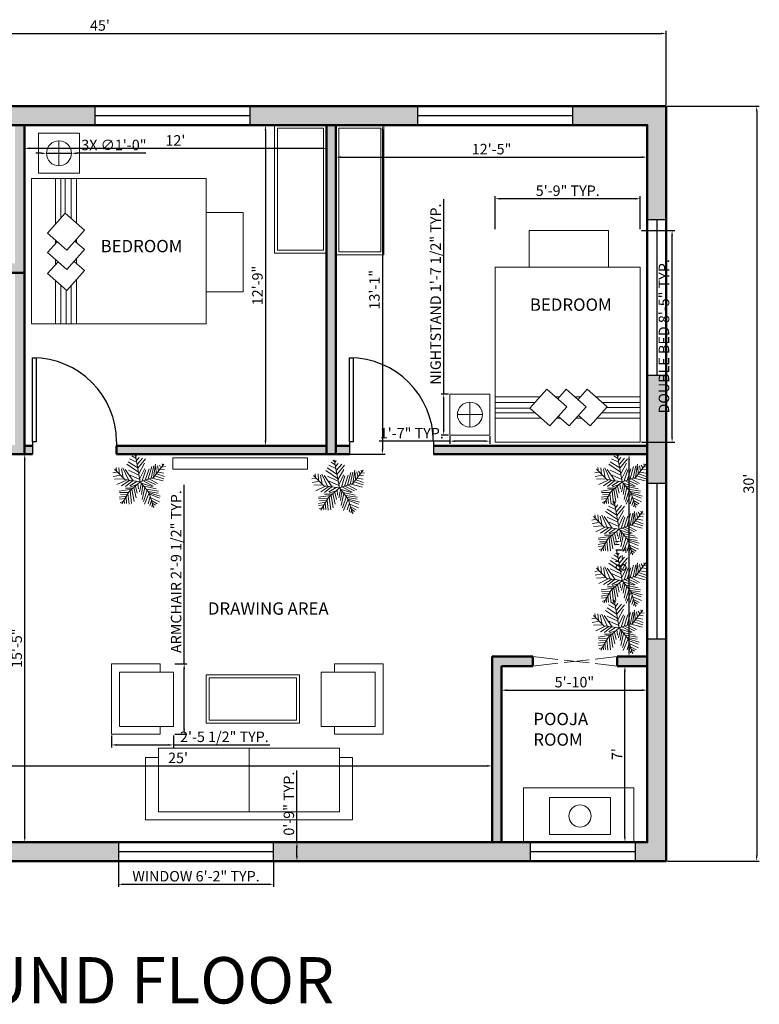
# Model space of a CAD drawing. Units: inches. Extents: x 1882 to 2467, y 1298 to 1767.
# Tile 2 of 2: x 2114 to 2467, y 1298 to 1767. Entities that reach past the tile are written whole.
import ezdxf

# ---------------------------------------------------------------- set-up
doc = ezdxf.new("R2010")
doc.units = ezdxf.units.IN
doc.linetypes.add('ACAD_ISO02W100', pattern=[15, 12, -3])
for name, color, linetype, lineweight in [('A-ANNO-DIMS', 2, 'Continuous', 18), ('A-ANNO-TEXT', 7, 'Continuous', 35), ('A-AREA-IDEN', 7, 'Continuous', 25), ('A-FURN', 8, 'Continuous', 18), ('A-WALL-OVHD', 160, 'ACAD_ISO02W100', 18), ('A-WALL-PATT', 160, 'Continuous', 13), ('DOOR', 140, 'Continuous', 25), ('TREE', 80, 'Continuous', 13), ('WALL', 160, 'Continuous', 50), ('WIND', 52, 'Continuous', 25)]:
    doc.layers.add(name, color=color, linetype=linetype, lineweight=lineweight)
doc.styles.get("Standard").update_dxf_attribs({"font": 'arial.ttf'})
doc.dimstyles.new('ISO-25', dxfattribs={"dimtxt": 5, "dimasz": 2.5, "dimexe": 1.25, "dimexo": 0.625, "dimtad": 1, "dimdec": 0, "dimlunit": 4, "dimtxsty": 'Standard', "dimcen": 2.5, "dimadec": 0, "dimazin": 0, "dimtfac": 1, "dimtdec": 0, "dimtmove": 0, "dimatfit": 3, "dimfxl": 1, "dimarcsym": 0})

# ---------------------------------------------------------------- blocks, each defined once
blk = doc.blocks.new('*U2')
for p, q in [((0, 0), (0, -6)), ((40, 0), (40, -6))]:
    blk.add_line(p, q)
blk.add_lwpolyline([(0, 0), (0, 40), (1.75, 40), (1.75, 0)], close=True)
blk.add_arc((0, 0), 40, 0, 90)
blk = doc.blocks.new('*D11')
at = {"layer": 'A-ANNO-DIMS', "color": 0, "lineweight": -2, "transparency": 16777216}
for p, q in [((2116.22, 1716.45), (2116.22, 1704.74)), ((2260.22, 1716.45), (2260.22, 1704.74)), ((2118.72, 1705.99), (2257.72, 1705.99))]:
    blk.add_line(p, q, dxfattribs=at)
at = {"layer": 'A-ANNO-DIMS', "color": 0, "lineweight": 100, "transparency": 16777216}
for points in [[(2118.72, 1706.41), (2118.72, 1705.57), (2116.22, 1705.99)], [(2257.72, 1706.41), (2257.72, 1705.57), (2260.22, 1705.99)]]:
    blk.add_solid(points, dxfattribs=at)
at = {"layer": 'Defpoints', "color": 0, "lineweight": 100, "transparency": 16777216}
for p in [(2116.22, 1717.07), (2260.22, 1717.07), (2260.22, 1705.99)]:
    blk.add_point(p, dxfattribs=at)
at = {"layer": 'A-ANNO-DIMS', "color": 0, "transparency": 16777216, "insert": (2188.22, 1709.12), "char_height": 5, "attachment_point": 5}
blk.add_mtext("12'", dxfattribs=at)
blk = doc.blocks.new('*D12')
at = {"layer": 'A-ANNO-DIMS', "color": 0, "lineweight": -2, "transparency": 16777216}
for p, q in [((2259.59, 1717.07), (2229.92, 1717.07)), ((2231.17, 1714.57), (2231.17, 1566.57)), ((2259.59, 1564.07), (2229.92, 1564.07))]:
    blk.add_line(p, q, dxfattribs=at)
at = {"layer": 'A-ANNO-DIMS', "color": 0, "lineweight": 100, "transparency": 16777216}
for points in [[(2230.75, 1714.57), (2231.58, 1714.57), (2231.17, 1717.07)], [(2230.75, 1566.57), (2231.58, 1566.57), (2231.17, 1564.07)]]:
    blk.add_solid(points, dxfattribs=at)
at = {"layer": 'Defpoints', "color": 0, "lineweight": 100, "transparency": 16777216}
for p in [(2260.22, 1717.07), (2231.17, 1564.07), (2260.22, 1564.07)]:
    blk.add_point(p, dxfattribs=at)
at = {"layer": 'A-ANNO-DIMS', "color": 0, "transparency": 16777216, "insert": (2227.99, 1640.57), "char_height": 5, "attachment_point": 5, "rotation": 90}
blk.add_mtext('12\'-9"', dxfattribs=at)
blk = doc.blocks.new('*D13')
at = {"layer": 'A-ANNO-DIMS', "color": 0, "lineweight": -2, "transparency": 16777216}
for p, q in [((2264.72, 1716.45), (2264.72, 1700.54)), ((2413.22, 1716.45), (2413.22, 1700.54)), ((2267.22, 1701.79), (2410.72, 1701.79))]:
    blk.add_line(p, q, dxfattribs=at)
at = {"layer": 'A-ANNO-DIMS', "color": 0, "lineweight": 100, "transparency": 16777216}
for points in [[(2267.22, 1702.21), (2267.22, 1701.38), (2264.72, 1701.79)], [(2410.72, 1702.21), (2410.72, 1701.38), (2413.22, 1701.79)]]:
    blk.add_solid(points, dxfattribs=at)
at = {"layer": 'Defpoints', "color": 0, "lineweight": 100, "transparency": 16777216}
for p in [(2264.72, 1717.07), (2413.22, 1717.07), (2413.22, 1701.79)]:
    blk.add_point(p, dxfattribs=at)
at = {"layer": 'A-ANNO-DIMS', "color": 0, "transparency": 16777216, "insert": (2338.97, 1704.97), "char_height": 5, "attachment_point": 5}
blk.add_mtext('12\'-5"', dxfattribs=at)
blk = doc.blocks.new('*D14')
at = {"layer": 'A-ANNO-DIMS', "color": 0, "lineweight": -2, "transparency": 16777216}
for p, q in [((2265.34, 1717.07), (2288.2, 1717.07)), ((2286.95, 1714.57), (2286.95, 1562.57)), ((2265.34, 1560.07), (2288.2, 1560.07))]:
    blk.add_line(p, q, dxfattribs=at)
at = {"layer": 'A-ANNO-DIMS', "color": 0, "lineweight": 100, "transparency": 16777216}
for points in [[(2286.53, 1714.57), (2287.36, 1714.57), (2286.95, 1717.07)], [(2286.53, 1562.57), (2287.36, 1562.57), (2286.95, 1560.07)]]:
    blk.add_solid(points, dxfattribs=at)
at = {"layer": 'Defpoints', "color": 0, "lineweight": 100, "transparency": 16777216}
for p in [(2264.72, 1717.07), (2264.72, 1560.07), (2286.95, 1560.07)]:
    blk.add_point(p, dxfattribs=at)
at = {"layer": 'A-ANNO-DIMS', "color": 0, "transparency": 16777216, "insert": (2283.77, 1638.57), "char_height": 5, "attachment_point": 5, "rotation": 90}
blk.add_mtext('13\'-1"', dxfattribs=at)
blk = doc.blocks.new('*D15')
at = {"layer": 'A-ANNO-DIMS', "color": 0, "lineweight": -2, "transparency": 16777216}
for p, q in [((2343.72, 1458.45), (2343.72, 1446.31)), ((2413.22, 1458.45), (2413.22, 1446.31)), ((2346.22, 1447.56), (2410.72, 1447.56))]:
    blk.add_line(p, q, dxfattribs=at)
at = {"layer": 'A-ANNO-DIMS', "color": 0, "lineweight": 100, "transparency": 16777216}
for points in [[(2346.22, 1447.98), (2346.22, 1447.14), (2343.72, 1447.56)], [(2410.72, 1447.98), (2410.72, 1447.14), (2413.22, 1447.56)]]:
    blk.add_solid(points, dxfattribs=at)
at = {"layer": 'Defpoints', "color": 0, "lineweight": 100, "transparency": 16777216}
for p in [(2343.72, 1459.07), (2413.22, 1459.07), (2413.22, 1447.56)]:
    blk.add_point(p, dxfattribs=at)
at = {"layer": 'A-ANNO-DIMS', "color": 0, "transparency": 16777216, "insert": (2378.47, 1450.74), "char_height": 5, "attachment_point": 5}
blk.add_mtext('5\'-10"', dxfattribs=at)
blk = doc.blocks.new('*D16')
at = {"layer": 'A-ANNO-DIMS', "color": 0, "lineweight": -2, "transparency": 16777216}
for p, q in [((2412.59, 1459.07), (2401.3, 1459.07)), ((2402.55, 1377.57), (2402.55, 1456.57)), ((2412.59, 1375.07), (2401.3, 1375.07))]:
    blk.add_line(p, q, dxfattribs=at)
at = {"layer": 'A-ANNO-DIMS', "color": 0, "lineweight": 100, "transparency": 16777216}
for points in [[(2402.13, 1456.57), (2402.97, 1456.57), (2402.55, 1459.07)], [(2402.13, 1377.57), (2402.97, 1377.57), (2402.55, 1375.07)]]:
    blk.add_solid(points, dxfattribs=at)
at = {"layer": 'Defpoints', "color": 0, "lineweight": 100, "transparency": 16777216}
for p in [(2402.55, 1459.07), (2413.22, 1459.07), (2413.22, 1375.07)]:
    blk.add_point(p, dxfattribs=at)
at = {"layer": 'A-ANNO-DIMS', "color": 0, "transparency": 16777216, "insert": (2399.42, 1417.07), "char_height": 5, "attachment_point": 5, "rotation": 90}
blk.add_mtext("7'", dxfattribs=at)
blk = doc.blocks.new('*D17')
at = {"layer": 'A-ANNO-DIMS', "color": 0, "lineweight": -2, "transparency": 16777216}
for p, q in [((2039.72, 1375.7), (2039.72, 1412.69)), ((2042.22, 1411.44), (2336.72, 1411.44)), ((2339.22, 1375.7), (2339.22, 1412.69))]:
    blk.add_line(p, q, dxfattribs=at)
at = {"layer": 'A-ANNO-DIMS', "color": 0, "lineweight": 100, "transparency": 16777216}
for points in [[(2042.22, 1411.86), (2042.22, 1411.02), (2039.72, 1411.44)], [(2336.72, 1411.86), (2336.72, 1411.02), (2339.22, 1411.44)]]:
    blk.add_solid(points, dxfattribs=at)
at = {"layer": 'Defpoints', "color": 0, "lineweight": 100, "transparency": 16777216}
for p in [(2339.22, 1411.44), (2039.72, 1375.07), (2339.22, 1375.07)]:
    blk.add_point(p, dxfattribs=at)
at = {"layer": 'A-ANNO-DIMS', "color": 0, "transparency": 16777216, "insert": (2189.47, 1414.62), "char_height": 5, "attachment_point": 5}
blk.add_mtext("25'", dxfattribs=at)
blk = doc.blocks.new('*D24')
at = {"layer": 'A-ANNO-DIMS', "color": 0, "lineweight": -2, "transparency": 16777216}
for p, q in [((2110.74, 1560.07), (2117.62, 1560.07)), ((2116.37, 1377.57), (2116.37, 1557.57)), ((2110.74, 1375.07), (2117.62, 1375.07))]:
    blk.add_line(p, q, dxfattribs=at)
at = {"layer": 'A-ANNO-DIMS', "color": 0, "lineweight": 100, "transparency": 16777216}
for points in [[(2115.96, 1557.57), (2116.79, 1557.57), (2116.37, 1560.07)], [(2115.96, 1377.57), (2116.79, 1377.57), (2116.37, 1375.07)]]:
    blk.add_solid(points, dxfattribs=at)
at = {"layer": 'Defpoints', "color": 0, "lineweight": 100, "transparency": 16777216}
for p in [(2110.11, 1560.07), (2116.37, 1560.07), (2110.11, 1375.07)]:
    blk.add_point(p, dxfattribs=at)
at = {"layer": 'A-ANNO-DIMS', "color": 0, "transparency": 16777216, "insert": (2113.2, 1467.57), "char_height": 5, "attachment_point": 5, "rotation": 90}
blk.add_mtext('15\'-5"', dxfattribs=at)
blk = doc.blocks.new('*D25')
at = {"layer": 'A-ANNO-DIMS', "color": 0, "lineweight": -2, "transparency": 16777216}
for p, q in [((2412.59, 1560.07), (2403.28, 1560.07)), ((2404.53, 1466.07), (2404.53, 1557.57)), ((2412.59, 1463.57), (2403.28, 1463.57))]:
    blk.add_line(p, q, dxfattribs=at)
at = {"layer": 'A-ANNO-DIMS', "color": 0, "lineweight": 100, "transparency": 16777216}
for points in [[(2404.12, 1557.57), (2404.95, 1557.57), (2404.53, 1560.07)], [(2404.12, 1466.07), (2404.95, 1466.07), (2404.53, 1463.57)]]:
    blk.add_solid(points, dxfattribs=at)
at = {"layer": 'Defpoints', "color": 0, "lineweight": 100, "transparency": 16777216}
for p in [(2404.53, 1560.07), (2413.22, 1560.07), (2413.22, 1463.57)]:
    blk.add_point(p, dxfattribs=at)
at = {"layer": 'A-ANNO-DIMS', "color": 0, "transparency": 16777216, "insert": (2401.35, 1511.82), "char_height": 5, "attachment_point": 5, "rotation": 90}
blk.add_mtext('8\'-1"', dxfattribs=at)
blk = doc.blocks.new('*D26')
at = {"layer": 'A-ANNO-DIMS', "color": 0, "lineweight": -2, "transparency": 16777216}
for p, q in [((1882.22, 1726.7), (1882.22, 1762.02)), ((2422.22, 1726.7), (2422.22, 1762.02)), ((1884.72, 1760.77), (2419.72, 1760.77))]:
    blk.add_line(p, q, dxfattribs=at)
at = {"layer": 'A-ANNO-DIMS', "color": 0, "lineweight": 100, "transparency": 16777216}
for points in [[(1884.72, 1761.18), (1884.72, 1760.35), (1882.22, 1760.77)], [(2419.72, 1761.18), (2419.72, 1760.35), (2422.22, 1760.77)]]:
    blk.add_solid(points, dxfattribs=at)
at = {"layer": 'Defpoints', "color": 0, "lineweight": 100, "transparency": 16777216}
for p in [(2422.22, 1760.77), (1882.22, 1726.07), (2422.22, 1726.07)]:
    blk.add_point(p, dxfattribs=at)
at = {"layer": 'A-ANNO-DIMS', "color": 0, "transparency": 16777216, "insert": (2152.22, 1763.93), "char_height": 5, "attachment_point": 5}
blk.add_mtext("45'", dxfattribs=at)
blk = doc.blocks.new('*D27')
at = {"layer": 'A-ANNO-DIMS', "color": 0, "lineweight": -2, "transparency": 16777216}
for p, q in [((2422.84, 1726.07), (2466.63, 1726.07)), ((2465.38, 1723.57), (2465.38, 1368.57)), ((2422.84, 1366.07), (2466.63, 1366.07))]:
    blk.add_line(p, q, dxfattribs=at)
at = {"layer": 'A-ANNO-DIMS', "color": 0, "lineweight": 100, "transparency": 16777216}
for points in [[(2464.97, 1723.57), (2465.8, 1723.57), (2465.38, 1726.07)], [(2464.97, 1368.57), (2465.8, 1368.57), (2465.38, 1366.07)]]:
    blk.add_solid(points, dxfattribs=at)
at = {"layer": 'Defpoints', "color": 0, "lineweight": 100, "transparency": 16777216}
for p in [(2422.22, 1726.07), (2422.22, 1366.07), (2465.38, 1366.07)]:
    blk.add_point(p, dxfattribs=at)
at = {"layer": 'A-ANNO-DIMS', "color": 0, "transparency": 16777216, "insert": (2462.2, 1546.07), "char_height": 5, "attachment_point": 5, "rotation": 90}
blk.add_mtext("30'", dxfattribs=at)
blk = doc.blocks.new('*U6')
for p, q in [((-5.114, 28.097), (-24.676, 40.636)), ((-7.288, 39.707), (-21.778, 46.673)), ((-8.737, 47.138), (-17.069, 52.711)), ((-10.186, 53.64), (-13.084, 55.962)), ((0, 0), (-10.5, 57)), ((-9.099, 51.782), (-6.563, 55.962)), ((-7.65, 43.423), (-2.578, 49.46)), ((-5.839, 35.992), (4.667, 48.067)), ((-5.114, 27.632), (10.463, 46.673)), ((-31.5, 4.5), (-52.5, 25.5)), ((-48.585, 21.131), (-49.309, 29.026)), ((-43.513, 28.561), (-42.427, 15.558)), ((-38.442, 26.239), (-34.819, 7.663)), ((-35.544, 28.097), (-24.314, 3.947)), ((-14.533, 2.09), (-30.834, 25.31)), ((-3.665, 19.273), (-27.574, 35.527)), ((-24.314, 23.917), (-2.941, 13.7)), ((-2.941, 16.486), (8.652, 37.85)), ((-1.129, 6.734), (9.014, 26.704)), ((3.942, 1.625), (11.187, 24.381)), ((10.101, 3.483), (17.708, 26.239)), ((16.259, 5.805), (23.142, 31.348)), ((22.055, 7.198), (27.489, 32.277)), ((27, 9), (48, 36)), ((27.127, 9.056), (31.112, 35.992)), ((31.836, 30.883), (32.561, 16.486)), ((35.096, 32.741), (37.27, 22.524)), ((38.719, 34.134), (41.979, 28.561)), ((40.53, 25.775), (48.862, 24.846)), ((43.791, 29.954), (51.036, 30.883)), ((44.153, 36.456), (45.239, 32.741)), ((-47.498, 19.737), (-55.83, 18.344)), ((-40.615, 13.7), (-55.105, 10.913)), ((-33.37, 6.269), (-52.207, 5.34)), ((-28.299, 3.483), (-47.86, -5.805)), ((-21.416, 3.018), (-38.079, -8.128)), ((0, 0), (-31.5, 4.5)), ((-15.982, 2.09), (-30.11, -9.521)), ((0, 0), (-22.5, -19.5)), ((-6.563, 1.161), (-21.416, -8.128)), ((-20.691, 13.7), (-1.129, 4.876)), ((0, 0), (27, 9)), ((0, 0), (18, -22.5)), ((6.478, 1.625), (26.04, -8.592)), ((11.187, 3.483), (30.749, -5.805)), ((18.07, 5.805), (35.096, -3.483)), ((24.229, 7.663), (46.688, 1.625)), ((29.662, 12.307), (48.137, 6.269)), ((33.285, 16.486), (48.862, 10.913)), ((36.183, 19.737), (48.137, 17.88)), ((-17.431, -15.094), (-42.789, -18.809)), ((-22.5, -19.5), (-37.5, -45)), ((-15.257, -12.772), (-30.11, -12.772)), ((-20.691, -18.345), (-17.793, -44.352)), ((-6.563, -5.805), (-19.967, -9.985)), ((-17.069, -15.094), (-12.721, -40.172)), ((-13.446, -11.378), (-8.737, -32.741)), ((-9.461, -8.592), (-6.201, -23.453)), ((-4.752, -3.483), (-3.665, -14.629)), ((2.493, -3.019), (-1.491, -20.202)), ((1.769, -2.555), (24.229, -9.521)), ((5.029, -6.27), (2.131, -25.775)), ((9.014, -11.378), (3.58, -35.992)), ((14.085, -16.951), (6.478, -40.172)), ((7.565, -9.056), (32.198, -14.629)), ((12.274, -15.094), (36.907, -18.809)), ((16.259, -19.738), (36.183, -22.989)), ((-28.299, -29.026), (-42.789, -31.348)), ((-24.314, -21.596), (-42.427, -22.06)), ((-30.834, -34.135), (-42.427, -35.528)), ((-34.457, -39.708), (-40.978, -42.494)), ((-26.849, -26.24), (-40.253, -25.775)), ((-32.646, -36.921), (-31.921, -44.352)), ((-29.023, -30.884), (-27.936, -43.887)), ((-25.038, -23.918), (-22.865, -45.281)), ((18.07, -22.524), (8.289, -45.745)), ((20.244, -30.419), (15.897, -44.816)), ((18, -22.5), (27, -52.5)), ((18.433, -22.524), (40.53, -29.026)), ((19.157, -25.311), (38.719, -33.206)), ((22.78, -37.85), (19.519, -48.532)), ((21.331, -32.741), (39.081, -40.636)), ((22.78, -38.314), (34.372, -44.816)), ((24.591, -45.745), (23.142, -50.854)), ((24.591, -43.423), (30.749, -47.603)), ((26.764, -49.925), (28.213, -50.854))]:
    blk.add_line(p, q)
blk = doc.blocks.new('WIN-74IN')
blk.add_line((0, 4.5), (74.03, 4.5))
blk.add_lwpolyline([(0, 0), (74.03, 0), (74.03, 9), (0, 9)], close=True)
blk = doc.blocks.new('BED-DOUBLE')
for p, q in [((11.49, 47.34), (11.49, 69.21)), ((14, 50.17), (14, 69.21)), ((16.17, 52.63), (16.17, 69.21)), ((18.98, 50.15), (18.98, 69.21)), ((21.58, 47.84), (21.58, 69.21)), ((11.49, 38.12), (11.49, 39.83)), ((21.58, 38.62), (21.58, 40.3)), ((11.49, 28.1), (11.49, 30.61)), ((21.58, 28.61), (21.58, 31.07)), ((11.49, 0), (11.49, 20.59)), ((21.58, 0), (21.58, 21.06)), ((14, 0), (14, 18.37)), ((16.55, 0), (16.55, 16.12)), ((18.98, 0), (18.98, 18.12))]:
    blk.add_line(p, q)
for points in [[(0, 69.21), (83.41, 69.21), (83.41, 0), (0, 0)], [(7.76, 43.13), (16.17, 52.63), (25.33, 44.53), (16.92, 35.02)], [(83.41, 15.22), (100.98, 15.22), (100.98, 53.07), (83.41, 53.07)]]:
    blk.add_lwpolyline(points, close=True)
for points in [[(20.75, 39.36), (25.33, 35.3), (16.92, 25.8), (7.76, 33.9), (12.34, 39.08)], [(20.36, 29.69), (25.33, 25.29), (16.92, 15.79), (7.76, 23.89), (12.73, 29.51)]]:
    blk.add_lwpolyline(points)
blk = doc.blocks.new('NIGHTSTAND-LAMP')
for p, q in [((9.73, 9.55), (9.73, 15.52)), ((9.73, 15.52), (9.73, 3.59)), ((15.7, 9.55), (3.77, 9.55)), ((9.73, 3.59), (9.73, 9.55)), ((9.73, 9.55), (15.7, 9.55))]:
    blk.add_line(p, q)
blk.add_lwpolyline([(0, 0), (19.47, 0), (19.47, 19.1), (0, 19.1)], close=True)
blk.add_circle((9.73, 9.55), 5.97)
blk = doc.blocks.new('ARMCHAIR')
for p, q in [((0, 0), (0, 33.67)), ((0, 33.67), (23.2, 33.67)), ((23.2, 33.67), (23.2, 29.68)), ((23.2, 0), (0, 0)), ((23.2, 3.77), (23.2, 0))]:
    blk.add_line(p, q)
blk.add_lwpolyline([(29.66, 3.77), (3.9, 3.77), (3.9, 29.68), (29.66, 29.68)], close=True)
blk = doc.blocks.new('*D33')
at = {"layer": 'A-ANNO-DIMS', "color": 0, "lineweight": -2, "transparency": 16777216}
for p, q in [((2161.01, 1365.45), (2161.01, 1353.72)), ((2235.04, 1365.45), (2235.04, 1353.72)), ((2163.51, 1354.97), (2232.54, 1354.97))]:
    blk.add_line(p, q, dxfattribs=at)
at = {"layer": 'A-ANNO-DIMS', "color": 0, "lineweight": 100, "transparency": 16777216}
for points in [[(2163.51, 1355.39), (2163.51, 1354.55), (2161.01, 1354.97)], [(2232.54, 1355.39), (2232.54, 1354.55), (2235.04, 1354.97)]]:
    blk.add_solid(points, dxfattribs=at)
at = {"layer": 'Defpoints', "color": 0, "lineweight": 100, "transparency": 16777216}
for p in [(2161.01, 1366.07), (2235.04, 1366.07), (2235.04, 1354.97)]:
    blk.add_point(p, dxfattribs=at)
at = {"layer": 'A-ANNO-DIMS', "color": 0, "transparency": 16777216, "insert": (2198.02, 1358.18), "char_height": 5, "attachment_point": 5}
blk.add_mtext('WINDOW 6\'-2" TYP.', dxfattribs=at)
blk = doc.blocks.new('*D34')
at = {"layer": 'A-ANNO-DIMS', "color": 0, "lineweight": -2, "transparency": 16777216}
for p, q in [((2246.15, 1375.07), (2246.15, 1409.3)), ((2235.67, 1375.07), (2247.4, 1375.07)), ((2246.15, 1368.57), (2246.15, 1372.57)), ((2235.67, 1366.07), (2247.4, 1366.07))]:
    blk.add_line(p, q, dxfattribs=at)
at = {"layer": 'A-ANNO-DIMS', "color": 0, "lineweight": 100, "transparency": 16777216}
for points in [[(2245.73, 1372.57), (2246.56, 1372.57), (2246.15, 1375.07)], [(2245.73, 1368.57), (2246.56, 1368.57), (2246.15, 1366.07)]]:
    blk.add_solid(points, dxfattribs=at)
at = {"layer": 'Defpoints', "color": 0, "lineweight": 100, "transparency": 16777216}
for p in [(2235.04, 1375.07), (2246.15, 1375.07), (2235.04, 1366.07)]:
    blk.add_point(p, dxfattribs=at)
at = {"layer": 'A-ANNO-DIMS', "color": 0, "transparency": 16777216, "insert": (2242.97, 1393.44), "char_height": 5, "attachment_point": 5, "rotation": 90}
blk.add_mtext('0\'-9" TYP.', dxfattribs=at)
blk = doc.blocks.new('*D37')
at = {"layer": 'A-ANNO-DIMS', "color": 0, "lineweight": -2, "transparency": 16777216}
for p, q in [((2410.51, 1666.81), (2426.29, 1666.81)), ((2425.04, 1568.33), (2425.04, 1664.31)), ((2410.51, 1565.83), (2426.29, 1565.83))]:
    blk.add_line(p, q, dxfattribs=at)
at = {"layer": 'A-ANNO-DIMS', "color": 0, "lineweight": 100, "transparency": 16777216}
for points in [[(2424.62, 1664.31), (2425.45, 1664.31), (2425.04, 1666.81)], [(2424.62, 1568.33), (2425.45, 1568.33), (2425.04, 1565.83)]]:
    blk.add_solid(points, dxfattribs=at)
at = {"layer": 'Defpoints', "color": 0, "lineweight": 100, "transparency": 16777216}
for p in [(2409.89, 1666.81), (2425.04, 1666.81), (2409.89, 1565.83)]:
    blk.add_point(p, dxfattribs=at)
at = {"layer": 'A-ANNO-DIMS', "color": 0, "transparency": 16777216, "insert": (2421.82, 1616.32), "char_height": 5, "attachment_point": 5, "rotation": 90}
blk.add_mtext('DOUBLE BED 8\'-5" TYP.', dxfattribs=at)
blk = doc.blocks.new('*D38')
at = {"layer": 'A-ANNO-DIMS', "color": 0, "lineweight": -2, "transparency": 16777216}
for p, q in [((2340.68, 1667.44), (2340.68, 1683.21)), ((2407.39, 1681.96), (2343.18, 1681.96)), ((2409.89, 1667.44), (2409.89, 1683.21))]:
    blk.add_line(p, q, dxfattribs=at)
at = {"layer": 'A-ANNO-DIMS', "color": 0, "lineweight": 100, "transparency": 16777216}
for points in [[(2343.18, 1682.38), (2343.18, 1681.54), (2340.68, 1681.96)], [(2407.39, 1682.38), (2407.39, 1681.54), (2409.89, 1681.96)]]:
    blk.add_solid(points, dxfattribs=at)
at = {"layer": 'Defpoints', "color": 0, "lineweight": 100, "transparency": 16777216}
for p in [(2340.68, 1681.96), (2340.68, 1666.81), (2409.89, 1666.81)]:
    blk.add_point(p, dxfattribs=at)
at = {"layer": 'A-ANNO-DIMS', "color": 0, "transparency": 16777216, "insert": (2375.29, 1685.14), "char_height": 5, "attachment_point": 5}
blk.add_mtext('5\'-9" TYP.', dxfattribs=at)
blk = doc.blocks.new('*D39')
at = {"layer": 'A-ANNO-DIMS', "color": 0, "lineweight": -2, "transparency": 16777216}
for p, q in [((2316.15, 1588.73), (2316.15, 1681.71)), ((2318.45, 1588.73), (2314.9, 1588.73)), ((2316.15, 1571.76), (2316.15, 1586.23)), ((2318.45, 1569.26), (2314.9, 1569.26))]:
    blk.add_line(p, q, dxfattribs=at)
at = {"layer": 'A-ANNO-DIMS', "color": 0, "lineweight": 100, "transparency": 16777216}
for points in [[(2315.74, 1586.23), (2316.57, 1586.23), (2316.15, 1588.73)], [(2315.74, 1571.76), (2316.57, 1571.76), (2316.15, 1569.26)]]:
    blk.add_solid(points, dxfattribs=at)
at = {"layer": 'Defpoints', "color": 0, "lineweight": 100, "transparency": 16777216}
for p in [(2316.15, 1588.73), (2319.07, 1588.73), (2319.07, 1569.26)]:
    blk.add_point(p, dxfattribs=at)
at = {"layer": 'A-ANNO-DIMS', "color": 0, "transparency": 16777216, "insert": (2312.94, 1636.47), "char_height": 5, "attachment_point": 5, "rotation": 90}
blk.add_mtext('NIGHTSTAND 1\'-7 1/2" TYP.', dxfattribs=at)
blk = doc.blocks.new('*D40')
at = {"layer": 'A-ANNO-DIMS', "color": 0, "lineweight": -2, "transparency": 16777216}
for p, q in [((2319.07, 1568.64), (2319.07, 1565.09)), ((2338.18, 1568.64), (2338.18, 1565.09)), ((2319.07, 1566.34), (2285.32, 1566.34)), ((2335.68, 1566.34), (2321.57, 1566.34))]:
    blk.add_line(p, q, dxfattribs=at)
at = {"layer": 'A-ANNO-DIMS', "color": 0, "lineweight": 100, "transparency": 16777216}
for points in [[(2321.57, 1566.76), (2321.57, 1565.93), (2319.07, 1566.34)], [(2335.68, 1566.76), (2335.68, 1565.93), (2338.18, 1566.34)]]:
    blk.add_solid(points, dxfattribs=at)
at = {"layer": 'Defpoints', "color": 0, "lineweight": 100, "transparency": 16777216}
for p in [(2319.07, 1569.26), (2338.18, 1569.26), (2319.07, 1566.34)]:
    blk.add_point(p, dxfattribs=at)
at = {"layer": 'A-ANNO-DIMS', "color": 0, "transparency": 16777216, "insert": (2300.95, 1569.48), "char_height": 5, "attachment_point": 5}
blk.add_mtext('1\'-7" TYP.', dxfattribs=at)
blk = doc.blocks.new('*D41')
at = {"layer": 'A-ANNO-DIMS', "color": 0, "lineweight": -2, "transparency": 16777216}
for p, q in [((2192.4, 1460.18), (2192.4, 1545.54)), ((2187.97, 1460.18), (2193.65, 1460.18)), ((2192.4, 1429.01), (2192.4, 1457.68)), ((2187.97, 1426.51), (2193.65, 1426.51))]:
    blk.add_line(p, q, dxfattribs=at)
at = {"layer": 'A-ANNO-DIMS', "color": 0, "lineweight": 100, "transparency": 16777216}
for points in [[(2191.98, 1457.68), (2192.82, 1457.68), (2192.4, 1460.18)], [(2191.98, 1429.01), (2192.82, 1429.01), (2192.4, 1426.51)]]:
    blk.add_solid(points, dxfattribs=at)
at = {"layer": 'Defpoints', "color": 0, "lineweight": 100, "transparency": 16777216}
for p in [(2187.35, 1460.18), (2192.4, 1460.18), (2187.35, 1426.51)]:
    blk.add_point(p, dxfattribs=at)
at = {"layer": 'A-ANNO-DIMS', "color": 0, "transparency": 16777216, "insert": (2189.19, 1504.11), "char_height": 5, "attachment_point": 5, "rotation": 90}
blk.add_mtext('ARMCHAIR 2\'-9 1/2" TYP.', dxfattribs=at)
blk = doc.blocks.new('*D42')
at = {"layer": 'A-ANNO-DIMS', "color": 0, "lineweight": -2, "transparency": 16777216}
for p, q in [((2157.68, 1425.88), (2157.68, 1420.21)), ((2187.35, 1425.88), (2187.35, 1420.21)), ((2160.18, 1421.46), (2184.85, 1421.46)), ((2187.35, 1421.46), (2233.31, 1421.46))]:
    blk.add_line(p, q, dxfattribs=at)
at = {"layer": 'A-ANNO-DIMS', "color": 0, "lineweight": 100, "transparency": 16777216}
for points in [[(2160.18, 1421.87), (2160.18, 1421.04), (2157.68, 1421.46)], [(2184.85, 1421.87), (2184.85, 1421.04), (2187.35, 1421.46)]]:
    blk.add_solid(points, dxfattribs=at)
at = {"layer": 'Defpoints', "color": 0, "lineweight": 100, "transparency": 16777216}
for p in [(2157.68, 1426.51), (2187.35, 1426.51), (2187.35, 1421.46)]:
    blk.add_point(p, dxfattribs=at)
at = {"layer": 'A-ANNO-DIMS', "color": 0, "transparency": 16777216, "insert": (2211.58, 1424.67), "char_height": 5, "attachment_point": 5}
blk.add_mtext('2\'-5 1/2" TYP.', dxfattribs=at)
blk = doc.blocks.new('*D43')
at = {"layer": 'A-ANNO-DIMS', "color": 0, "lineweight": -2, "transparency": 16777216}
for p, q in [((2124.22, 1703.62), (2121.72, 1703.62)), ((2126.72, 1703.62), (2138.65, 1703.62)), ((2174.11, 1703.62), (2141.15, 1703.62))]:
    blk.add_line(p, q, dxfattribs=at)
at = {"layer": 'A-ANNO-DIMS', "color": 0, "lineweight": 100, "transparency": 16777216}
for points in [[(2124.22, 1704.04), (2124.22, 1703.2), (2126.72, 1703.62)], [(2141.15, 1704.04), (2141.15, 1703.2), (2138.65, 1703.62)]]:
    blk.add_solid(points, dxfattribs=at)
at = {"layer": 'Defpoints', "color": 0, "lineweight": 100, "transparency": 16777216}
for p in [(2126.72, 1703.62), (2138.65, 1703.62)]:
    blk.add_point(p, dxfattribs=at)
at = {"layer": 'A-ANNO-DIMS', "color": 0, "transparency": 16777216, "insert": (2158.88, 1706.94), "char_height": 5, "attachment_point": 5, "rotation": 359.9995}
blk.add_mtext('3X ∅1\'-0"', dxfattribs=at)

msp = doc.modelspace()

# ---------------------------------------------------------------- hatches: boundary and pattern name
at = {"layer": 'A-WALL-PATT'}
h = msp.add_hatch(color=256, dxfattribs=at)
h.dxf.hatch_style = 1
h.paths.add_polyline_path([(1916.77, 1726.07), (1882.22, 1726.07), (1882.22, 1682.34), (1891.22, 1682.34), (1891.22, 1717.07), (1916.77, 1717.07)])
h.paths.add_polyline_path([(2064.04, 1726.07), (1990.8, 1726.07), (1990.8, 1717.07), (2035.22, 1717.07), (2064.04, 1717.07)])
h.paths.add_polyline_path([(2149.78, 1726.07), (2093.48, 1726.07), (2093.48, 1717.07), (2108.14, 1717.07), (2111.72, 1717.07), (2149.78, 1717.07)])
h.paths.add_polyline_path([(2116.22, 1717.07), (2111.72, 1717.07), (2111.72, 1651.07), (2039.72, 1651.07), (2039.72, 1646.57), (2116.22, 1646.57)])
h.paths.add_polyline_path([(2039.72, 1717.07), (2035.22, 1717.07), (2035.22, 1687.94), (2039.72, 1687.94)])
h.paths.add_polyline_path([(1891.22, 1608.31), (1882.22, 1608.31), (1882.22, 1537.91), (1891.22, 1537.91)])
h.paths.add_polyline_path([(2039.72, 1654.79), (2035.22, 1654.79), (2035.22, 1564.07), (2032.61, 1564.07), (2032.61, 1559.57), (2039.72, 1559.57)])
h.paths.add_polyline_path([(2043.01, 1592.08), (2043.01, 1564.25), (2041.79, 1564.25), (2041.79, 1592.11), (2043.01, 1592.11), (2043.01, 1592.08, -0.398105), (2069.65, 1564.57), (2111.72, 1564.57), (2111.72, 1646.57), (2116.22, 1646.57), (2116.22, 1560.07), (2069.65, 1560.07), (2069.65, 1564.25, 0.401453)])
h.paths.add_polyline_path([(2120.13, 1564.07), (2116.22, 1564.07), (2116.22, 1560.07), (2120.13, 1560.07)])
h.paths.add_polyline_path([(2271.23, 1564.07), (2264.72, 1564.07), (2264.72, 1560.07), (2271.23, 1560.07)])
h.paths.add_polyline_path([(2303.68, 1726.07), (2223.81, 1726.07), (2223.81, 1717.07), (2260.22, 1717.07), (2303.68, 1717.07)])
h.paths.add_polyline_path([(2422.22, 1726.07), (2377.71, 1726.07), (2377.71, 1717.07), (2413.22, 1717.07), (2413.22, 1671.81), (2422.22, 1671.81)])
h = msp.add_hatch(color=256, dxfattribs=at)
h.dxf.hatch_style = 1
h.paths.add_polyline_path([(2264.72, 1717.07), (2260.22, 1717.07), (2260.22, 1560.07), (2264.72, 1560.07)])
h.paths.add_polyline_path([(2260.22, 1564.07), (2160.13, 1564.07), (2160.13, 1560.07), (2260.22, 1560.07)])
h = msp.add_hatch(color=256, dxfattribs=at)
h.dxf.hatch_style = 1
h.paths.add_polyline_path([(2413.22, 1564.07), (2311.23, 1564.07), (2311.23, 1560.07), (2413.22, 1560.07)])
h.paths.add_polyline_path([(2422.22, 1597.77), (2413.22, 1597.77), (2413.22, 1546.07), (2422.22, 1546.07)])
h.paths.add_polyline_path([(2422.22, 1472.04), (2413.22, 1472.04), (2413.22, 1375.07), (2407.41, 1375.07), (2407.41, 1366.07), (2422.22, 1366.07)])
h.paths.add_polyline_path([(2343.72, 1459.07), (2358.61, 1459.07), (2358.61, 1463.57), (2339.22, 1463.57), (2339.22, 1375.07), (2343.72, 1375.07)])
h.paths.add_polyline_path([(2357.52, 1375.07), (2235.04, 1375.07), (2235.04, 1366.07), (2357.52, 1366.07)])
h.paths.add_polyline_path([(2413.22, 1463.57), (2398.81, 1463.57), (2398.81, 1459.07), (2413.22, 1459.07)])
h.paths.add_polyline_path([(2161.01, 1375.07), (2110.11, 1375.07), (2110.11, 1370.52), (2110.11, 1366.07), (2161.01, 1366.07)])
h.paths.add_polyline_path([(2050.88, 1375.07), (1999.86, 1375.07), (1999.86, 1366.07), (2050.88, 1366.07), (2050.88, 1370.52)])
h.paths.add_polyline_path([(2039.72, 1451.57), (2029.82, 1451.57), (2029.82, 1447.07), (2035.22, 1447.07), (2035.22, 1375.07), (2039.72, 1375.07)])
h.paths.add_polyline_path([(1891.22, 1399.07), (1891.22, 1463.87), (1882.22, 1463.87), (1882.22, 1366.07), (1925.83, 1366.07), (1925.83, 1375.07), (1891.22, 1375.07)])

# ---------------------------------------------------------------- linework, layer by layer
at = {"layer": 'A-FURN'}
for p, q in [((2223.37, 1419.95), (2223.37, 1389.56)), ((2180.22, 1415.43), (2173.97, 1415.43)), ((2173.97, 1415.43), (2173.97, 1385.72)), ((2180.22, 1415.43), (2180.22, 1415.43)), ((2272.62, 1415.43), (2266.53, 1415.43)), ((2272.62, 1385.72), (2272.62, 1415.43)), ((2173.97, 1385.72), (2272.62, 1385.72))]:
    msp.add_line(p, q, dxfattribs=at)
for points in [[(2260.22, 1717.07), (2235.51, 1717.07), (2235.51, 1656.01), (2260.22, 1656.01)], [(2258.78, 1715.64), (2236.95, 1715.64), (2236.95, 1657.45), (2258.78, 1657.45)], [(2264.72, 1655.24), (2287.54, 1655.24), (2287.54, 1717.07), (2264.72, 1717.07)], [(2266.15, 1656.68), (2286.1, 1656.68), (2286.1, 1715.64), (2266.15, 1715.64)], [(2187.04, 1558.33), (2251.28, 1558.33), (2251.28, 1553.05), (2187.04, 1553.05)], [(2202.93, 1454.88), (2247.34, 1454.88), (2247.34, 1431.81), (2202.93, 1431.81)], [(2204.37, 1453.44), (2245.9, 1453.44), (2245.9, 1433.25), (2204.37, 1433.25)], [(2180.22, 1389.56), (2266.53, 1389.56), (2266.53, 1419.95), (2180.22, 1419.95)], [(2354.26, 1375.07), (2406.84, 1375.07), (2406.84, 1400.92), (2354.26, 1400.92)], [(2366.58, 1378.79), (2395.71, 1378.79), (2395.71, 1396.33), (2366.58, 1396.33)]]:
    msp.add_lwpolyline(points, close=True, dxfattribs=at)
msp.add_circle((2381.14, 1387.56), 5.32, dxfattribs=at)
at = {"layer": 'A-WALL-OVHD'}
for p, q in [((2358.61, 1459.07), (2398.81, 1463.57)), ((2358.61, 1463.57), (2398.81, 1459.07))]:
    msp.add_line(p, q, dxfattribs=at)
at = {"layer": 'WALL'}
for p, q in [((1882.22, 1726.07), (2422.22, 1726.07)), ((2422.22, 1726.07), (2422.22, 1366.07)), ((2116.22, 1717.07), (2116.22, 1646.57)), ((2116.22, 1717.07), (2260.22, 1717.07)), ((2260.22, 1717.07), (2260.22, 1564.07)), ((2264.72, 1717.07), (2264.72, 1560.07)), ((2116.22, 1646.57), (2039.72, 1646.57)), ((2116.22, 1560.07), (2116.22, 1646.57)), ((2120.13, 1564.07), (2116.22, 1564.07)), ((2260.22, 1564.07), (2160.13, 1564.07)), ((2264.72, 1564.07), (2271.23, 1564.07)), ((2311.23, 1564.07), (2413.22, 1564.07)), ((2069.65, 1560.07), (2116.22, 1560.07)), ((2120.13, 1560.07), (2116.22, 1560.07)), ((2264.72, 1560.07), (2160.13, 1560.07)), ((2264.72, 1560.07), (2271.23, 1560.07)), ((2311.23, 1560.07), (2413.22, 1560.07)), ((2339.22, 1375.07), (2339.22, 1463.57)), ((2339.22, 1463.57), (2358.61, 1463.57)), ((2358.61, 1459.07), (2358.61, 1463.57)), ((2398.81, 1459.07), (2398.81, 1463.57)), ((2398.81, 1463.57), (2413.22, 1463.57)), ((2343.72, 1375.07), (2343.72, 1459.07)), ((2343.72, 1375.07), (2343.72, 1459.07)), ((2343.72, 1459.07), (2358.61, 1459.07)), ((2398.81, 1459.07), (2413.22, 1459.07)), ((2110.11, 1375.07), (2343.72, 1375.07)), ((2422.22, 1366.07), (2110.11, 1366.07))]:
    msp.add_line(p, q, dxfattribs=at)
for points in [[(2050.88, 1366.07), (1882.22, 1366.07), (1882.22, 1726.07), (2422.22, 1726.07), (2422.22, 1366.07), (2110.11, 1366.07)], [(2050.88, 1375.07), (1891.22, 1375.07), (1891.22, 1717.07), (2413.22, 1717.07), (2413.22, 1375.07), (2110.11, 1375.07)]]:
    msp.add_lwpolyline(points, dxfattribs=at)
for points in [[(2260.22, 1717.07), (2264.72, 1717.07), (2264.72, 1560.07), (2260.22, 1560.07)], [(2160.13, 1560.07), (2260.22, 1560.07), (2260.22, 1564.07), (2160.13, 1564.07)]]:
    msp.add_lwpolyline(points, close=True, dxfattribs=at)
at = {"layer": 'WIND'}
msp.add_line((2357.52, 1370.57), (2407.41, 1370.57), dxfattribs=at)
msp.add_lwpolyline([(2357.52, 1375.07), (2407.41, 1375.07), (2407.41, 1366.07), (2357.52, 1366.07)], close=True, dxfattribs=at)

# ---------------------------------------------------------------- block references
at = {"layer": 'A-FURN'}
for name, p in [('NIGHTSTAND-LAMP', (2122.95, 1694.07)), ('BED-DOUBLE', (2119.52, 1622.36)), ('ARMCHAIR', (2157.68, 1426.51))]:
    msp.add_blockref(name, p, dxfattribs=at)
for name, p, rotation in [('BED-DOUBLE', (2409.89, 1565.83), 89.99999999999991), ('NIGHTSTAND-LAMP', (2338.18, 1569.26), 90.00000000000198)]:
    msp.add_blockref(name, p, dxfattribs=dict(at, rotation=rotation))
at = {"layer": 'A-FURN', "extrusion": (0, 0, -1), "zscale": -1}
msp.add_blockref('ARMCHAIR', (-2287.32, 1426.51), dxfattribs=at)
at = {"layer": 'DOOR'}
for p in [(2120.13, 1566.07), (2271.23, 1566.07)]:
    msp.add_blockref('*U2', p, dxfattribs=at)
at = {"layer": 'TREE', "xscale": 0.234451498037333, "yscale": 0.234451498037333, "zscale": 0.234451498037333}
for p in [(2171.48, 1546.95), (2401.28, 1546.95), (2266.42, 1544.01), (2399.84, 1524.42), (2401.28, 1499.81), (2399.84, 1477.27)]:
    msp.add_blockref('*U6', p, dxfattribs=at)
at = {"layer": 'WIND'}
for p in [(2149.78, 1717.08), (2303.68, 1717.08), (2161.01, 1366.08)]:
    msp.add_blockref('WIN-74IN', p, dxfattribs=at)
for p, rotation in [((2413.22, 1671.81), 270), ((2413.22, 1546.07), 270.0000000000001)]:
    msp.add_blockref('WIN-74IN', p, dxfattribs=dict(at, rotation=rotation))

# ---------------------------------------------------------------- texts
at = {"layer": 'A-ANNO-TEXT', "insert": (2033.57, 1320.26), "char_height": 22.1185, "attachment_point": 1}
msp.add_mtext_dynamic_manual_height_columns('GROUND FLOOR', width=577.1514, gutter_width=110.59, heights=[0], dxfattribs=at)
at = {"layer": 'A-AREA-IDEN', "attachment_point": 1}
for s, insert, char_height in [('BEDROOM', (2152.54, 1662.31), 5.88), ('BEDROOM', (2357.23, 1634.38), 5.88), ('DRAWING AREA', (2203.7, 1489.45), 5.8799), ('POOJA \\PROOM', (2358.89, 1436.76), 5.88)]:
    msp.add_mtext_dynamic_manual_height_columns(s, width=153.4263, gutter_width=29.4, heights=[0], dxfattribs=dict(at, insert=insert, char_height=char_height))

# ---------------------------------------------------------------- dimensions: what is measured, and where the dimension line sits
at = {"layer": 'A-ANNO-DIMS'}
for base, p1, p2, picture, middle in [((2422.22, 1760.77), (1882.22, 1726.07), (2422.22, 1726.07), '*D26', (2152.22, 1763.93)), ((2260.22, 1705.99), (2116.22, 1717.07), (2260.22, 1717.07), '*D11', (2188.22, 1709.12)), ((2413.21873251, 1701.79408987), (2264.71873251, 1717.07458791), (2413.21873251, 1717.07458791), '*D13', (2338.96873251, 1704.97195481)), ((2413.21873251, 1447.55979488), (2343.71873251, 1459.07458791), (2413.21873251, 1459.07458791), '*D15', (2378.46873251, 1450.73765982)), ((2339.21873251, 1411.44158288), (2039.71873251, 1375.07458791), (2339.21873251, 1375.07458791), '*D17', (2189.46873251, 1414.61944782))]:
    dim = msp.add_linear_dim(base=base, p1=p1, p2=p2, dimstyle='ISO-25', override={"dimclrd": 0, "dimclre": 0, "dimclrt": 0}, dxfattribs=at)
    dim.commit()
    dim.dimension.update_dxf_attribs({"geometry": picture, "text_midpoint": middle})
for base, p1, p2, picture, middle in [((2465.38, 1366.07), (2422.22, 1726.07), (2422.22, 1366.07), '*D27', (2462.2, 1546.07)), ((2231.17, 1564.07), (2260.22, 1717.07), (2260.22, 1564.07), '*D12', (2227.99, 1640.57)), ((2286.95, 1560.07), (2264.72, 1717.07), (2264.72, 1560.07), '*D14', (2283.77, 1638.57)), ((2116.37, 1560.07), (2110.11, 1375.07), (2110.11, 1560.07), '*D24', (2113.2, 1467.57)), ((2404.53237276, 1560.07458791), (2413.21873251, 1463.57458791), (2413.21873251, 1560.07458791), '*D25', (2401.35450782, 1511.82458791)), ((2402.55, 1459.07), (2413.22, 1375.07), (2413.22, 1459.07), '*D16', (2399.42, 1417.07))]:
    dim = msp.add_linear_dim(base=base, p1=p1, p2=p2, angle=90, dimstyle='ISO-25', override={"dimclrd": 0, "dimclre": 0, "dimclrt": 0}, dxfattribs=at)
    dim.commit()
    dim.dimension.update_dxf_attribs({"geometry": picture, "text_midpoint": middle})
dim = msp.add_diameter_dim_2p(p1=(2126.72, 1703.62), p2=(2138.65, 1703.62), text='3X <>', dimstyle='ISO-25', override={"dimdec": 1, "dimlfac": 1, "dimrnd": 0, "dimzin": 1, "dimdsep": 46, "dimlunit": 4, "dimfrac": 2}, dxfattribs=at)
dim.commit()
dim.dimension.update_dxf_attribs({"geometry": '*D43', "text_midpoint": (2158.88, 1703.62), "dimtype": 163})
for base, p1, p2, angle, text, picture, middle in [((2340.68, 1681.96), (2409.89, 1666.81), (2340.68, 1666.81), 180, '<> TYP.', '*D38', (2375.29, 1685.14)), ((2316.15, 1588.73), (2319.07, 1569.26), (2319.07, 1588.73), 90, 'NIGHTSTAND <> TYP.', '*D39', (2312.94, 1636.47)), ((2425.04, 1666.81), (2409.89, 1565.83), (2409.89, 1666.81), 90, 'DOUBLE BED <> TYP.', '*D37', (2421.82, 1616.32)), ((2319.07, 1566.34), (2338.18, 1569.26), (2319.07, 1569.26), 180, '<> TYP.', '*D40', (2300.95, 1569.48)), ((2192.4, 1460.18), (2187.35, 1426.51), (2187.35, 1460.18), 90, 'ARMCHAIR <> TYP.', '*D41', (2189.19, 1504.11)), ((2246.15, 1375.07), (2235.04, 1366.07), (2235.04, 1375.07), 90, '<> TYP.', '*D34', (2242.97, 1393.44))]:
    dim = msp.add_linear_dim(base=base, p1=p1, p2=p2, angle=angle, text=text, dimstyle='ISO-25', override={"dimdec": 1, "dimlfac": 1, "dimrnd": 0, "dimzin": 1, "dimdsep": 46, "dimlunit": 4, "dimfrac": 2}, dxfattribs=at)
    dim.commit()
    dim.dimension.update_dxf_attribs({"geometry": picture, "text_midpoint": middle})
for base, p1, p2, text, picture, middle in [((2187.35, 1421.46), (2157.68, 1426.51), (2187.35, 1426.51), '<> TYP.', '*D42', (2211.58, 1424.67)), ((2235.04, 1354.97), (2161.01, 1366.07), (2235.04, 1366.07), 'WINDOW <> TYP.', '*D33', (2198.02, 1358.18))]:
    dim = msp.add_linear_dim(base=base, p1=p1, p2=p2, text=text, dimstyle='ISO-25', override={"dimdec": 1, "dimlfac": 1, "dimrnd": 0, "dimzin": 1, "dimdsep": 46, "dimlunit": 4, "dimfrac": 2}, dxfattribs=at)
    dim.commit()
    dim.dimension.update_dxf_attribs({"geometry": picture, "text_midpoint": middle})

doc.saveas('drawing.dxf')
